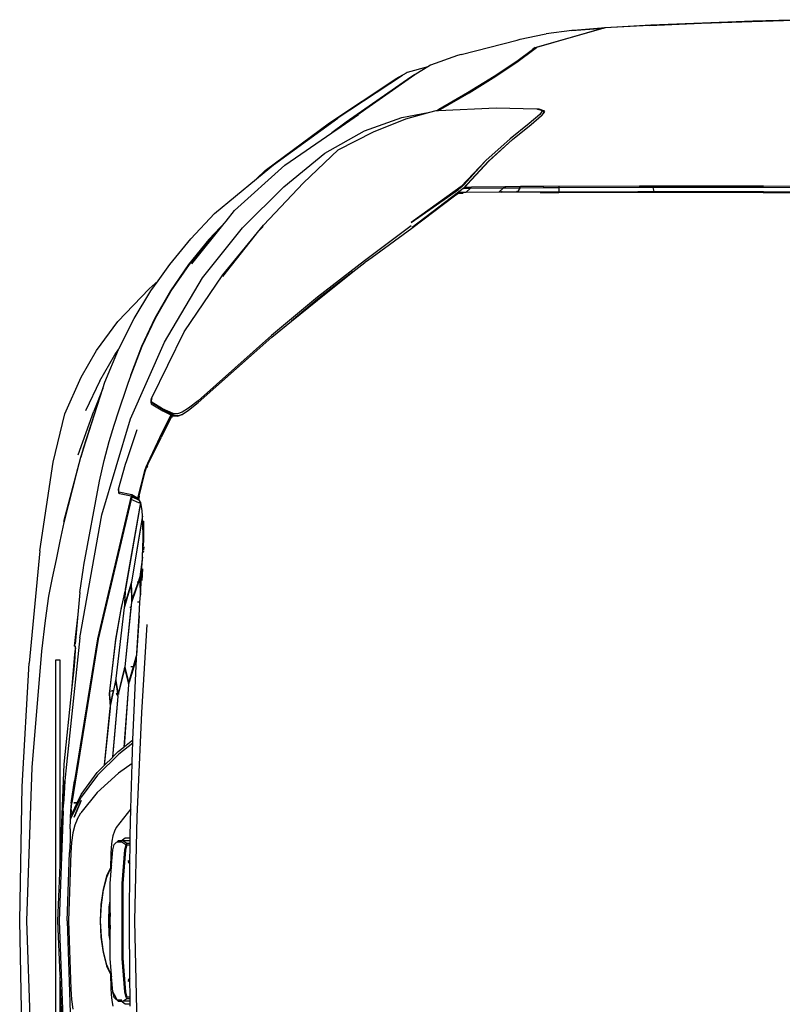
# Model space of a CAD drawing. Units: inches. Extents: x 22042254 to 25404563, y 17568978 to 17626777.
# Tile 12 of 45: x 22042340.5158 to 22042340.9867, y 17568978.1657 to 17568978.7735. Entities that reach past the tile are written whole.
import ezdxf

# ---------------------------------------------------------------- set-up
doc = ezdxf.new("R2010")
doc.units = ezdxf.units.IN
doc.header["$MEASUREMENT"] = 0
doc.layers.add('A-SITE-VEHI', color=8, linetype='Continuous', lineweight=18)
doc.layers.add('Edges', color=250, linetype='Continuous')

# ---------------------------------------------------------------- blocks, each defined once
blk = doc.blocks.new('Nissan Qashqai pl')
at = {"layer": 'Edges'}
for p, q in [((7.32157, 11.66208), (7.32157, 12.18208)), ((7.32607, 12.18208), (7.32607, 11.97794)), ((7.29801, 12.07497), (7.29279, 11.92208)), ((7.33017, 12.07853), (7.32607, 11.97794)), ((7.28835, 12.05625), (7.28572, 11.92208)), ((7.32507, 11.92208), (7.32911, 12.03155)), ((7.40018, 11.92208), (7.40245, 12.02601)), ((7.33294, 11.92208), (7.33653, 12.02372)), ((7.33733, 12.00038), (7.33865, 12.00996)), ((7.37751, 12.0015), (7.37864, 12.00699)), ((7.39589, 12.00706), (7.39588, 12.00508)), ((7.33667, 11.99003), (7.33733, 12.00038)), ((7.37683, 11.99537), (7.37751, 12.0015)), ((7.37985, 11.99831), (7.3787, 11.99283)), ((7.38081, 11.99933), (7.37985, 11.99831)), ((7.38074, 11.99908), (7.37985, 11.99831)), ((7.38002, 11.99534), (7.38305, 12.00106)), ((7.38074, 11.99908), (7.38081, 11.99933)), ((7.38104, 11.99933), (7.38074, 11.99908)), ((7.38081, 11.99933), (7.38402, 12.00208)), ((7.38104, 11.99933), (7.38081, 11.99933)), ((7.38305, 12.00106), (7.38104, 11.99933)), ((7.38659, 12.00106), (7.38305, 12.00106)), ((7.38402, 12.00208), (7.38696, 12.00208)), ((7.38683, 12.00198), (7.38659, 12.00106)), ((7.3875, 12.00106), (7.38659, 12.00106)), ((7.38696, 12.00208), (7.38683, 12.00198)), ((7.39094, 12.00508), (7.38696, 12.00208)), ((7.38696, 12.00208), (7.38847, 12.00208)), ((7.38847, 12.00208), (7.39254, 11.99933)), ((7.39551, 12.00208), (7.38847, 12.00208)), ((7.39041, 11.99283), (7.39156, 11.99831)), ((7.39564, 12.00508), (7.39094, 12.00508)), ((7.39288, 11.99808), (7.39173, 11.99259)), ((7.39254, 11.99933), (7.39582, 11.99933)), ((7.39254, 11.99933), (7.39288, 11.99808)), ((7.3958, 11.99808), (7.39288, 11.99808)), ((7.39551, 12.00208), (7.39584, 12.00183)), ((7.39588, 12.0049), (7.39564, 12.00508)), ((7.39588, 12.00508), (7.39564, 12.00508)), ((7.3958, 11.99808), (7.39564, 11.98012)), ((7.39582, 11.99933), (7.3958, 11.99808)), ((7.39584, 12.00183), (7.39582, 11.99933)), ((7.39588, 12.0049), (7.39584, 12.00183)), ((7.39588, 12.00508), (7.39588, 12.0049)), ((7.33429, 11.92208), (7.33667, 11.99003)), ((7.37614, 11.97511), (7.37648, 11.98901)), ((7.37648, 11.98901), (7.37683, 11.99537)), ((7.3787, 11.99283), (7.37743, 11.97775)), ((7.3787, 11.99283), (7.38002, 11.99534)), ((7.38759, 11.95948), (7.39041, 11.99283)), ((7.39173, 11.99259), (7.38892, 11.95935)), ((7.32607, 11.9764), (7.32607, 11.97794)), ((7.37614, 11.97511), (7.37686, 11.97673)), ((7.37686, 11.97673), (7.3771, 11.97702)), ((7.37713, 11.97709), (7.3771, 11.97702)), ((7.37743, 11.97775), (7.37713, 11.97709)), ((7.37713, 11.97709), (7.3774, 11.97738)), ((7.3774, 11.97738), (7.37727, 11.97594)), ((7.3774, 11.97738), (7.37743, 11.97775)), ((7.39385, 11.98229), (7.39564, 11.98012)), ((7.39563, 11.97885), (7.39385, 11.981)), ((7.39563, 11.97885), (7.3951, 11.92208)), ((7.39564, 11.98012), (7.39563, 11.97885)), ((7.32607, 11.9764), (7.3238, 11.92208)), ((7.37239, 11.9667), (7.37614, 11.97511)), ((7.37707, 11.97569), (7.37268, 11.96585)), ((7.37727, 11.97594), (7.37588, 11.95948)), ((7.37727, 11.97594), (7.37707, 11.97569)), ((7.36896, 11.95363), (7.37239, 11.9667)), ((7.37268, 11.96585), (7.36932, 11.95303)), ((7.37588, 11.95948), (7.37588, 11.94171)), ((7.38759, 11.88468), (7.38759, 11.95948)), ((7.38892, 11.95935), (7.38892, 11.88481)), ((7.36681, 11.93841), (7.36896, 11.95363)), ((7.36932, 11.95303), (7.3672, 11.9381)), ((7.36607, 11.92208), (7.36681, 11.93841)), ((7.3672, 11.9381), (7.36648, 11.92208)), ((7.37588, 11.94171), (7.37512, 11.93632)), ((7.37588, 11.94171), (7.37588, 11.93029)), ((7.37512, 11.93632), (7.37448, 11.92208)), ((7.37551, 11.92208), (7.37588, 11.93029)), ((7.37588, 11.93029), (7.37588, 11.91388)), ((7.28572, 11.92208), (7.28835, 11.78791)), ((7.29279, 11.92208), (7.29801, 11.76919)), ((7.3238, 11.92208), (7.32607, 11.86622)), ((7.32911, 11.81261), (7.32507, 11.92208)), ((7.33294, 11.92208), (7.33535, 11.85392)), ((7.33667, 11.85414), (7.33429, 11.92208)), ((7.36681, 11.90575), (7.36607, 11.92208)), ((7.36648, 11.92208), (7.3672, 11.90606)), ((7.37448, 11.92208), (7.37512, 11.90785)), ((7.37588, 11.91388), (7.37551, 11.92208)), ((7.3951, 11.92208), (7.39563, 11.86531)), ((7.40245, 11.81815), (7.40018, 11.92208)), ((7.37588, 11.91388), (7.37588, 11.90246)), ((7.36896, 11.89053), (7.36681, 11.90575)), ((7.3672, 11.90606), (7.36932, 11.89113)), ((7.37512, 11.90785), (7.37588, 11.90246)), ((7.37588, 11.90246), (7.37588, 11.88468)), ((7.37239, 11.87746), (7.36896, 11.89053)), ((7.36932, 11.89113), (7.37268, 11.87831)), ((7.37588, 11.88468), (7.37727, 11.86822)), ((7.39041, 11.85133), (7.38759, 11.88468)), ((7.38892, 11.88481), (7.39173, 11.85157)), ((7.37614, 11.86905), (7.37239, 11.87746)), ((7.37268, 11.87831), (7.37707, 11.86848)), ((7.37648, 11.85515), (7.37614, 11.86905)), ((7.37686, 11.86743), (7.37614, 11.86905)), ((7.32607, 11.86622), (7.33017, 11.76563)), ((7.32607, 11.86622), (7.32607, 11.66208)), ((7.3771, 11.86714), (7.37686, 11.86743)), ((7.37707, 11.86848), (7.37727, 11.86822)), ((7.3771, 11.86714), (7.37713, 11.86707)), ((7.37713, 11.86707), (7.37743, 11.86641)), ((7.3774, 11.86678), (7.37713, 11.86707)), ((7.37727, 11.86822), (7.3774, 11.86678)), ((7.3774, 11.86678), (7.37743, 11.86641)), ((7.37743, 11.86641), (7.3787, 11.85133)), ((7.39385, 11.86316), (7.39563, 11.86531)), ((7.39564, 11.86404), (7.39385, 11.86187)), ((7.39563, 11.86531), (7.39564, 11.86404)), ((7.39564, 11.86404), (7.3958, 11.84608)), ((7.33608, 11.84164), (7.33535, 11.85392)), ((7.33733, 11.84378), (7.33667, 11.85414)), ((7.37683, 11.8488), (7.37648, 11.85515)), ((7.3787, 11.85133), (7.37985, 11.84585)), ((7.39156, 11.84585), (7.39041, 11.85133)), ((7.39173, 11.85157), (7.39288, 11.84608)), ((7.33619, 11.83012), (7.33608, 11.84164)), ((7.33865, 11.8342), (7.33733, 11.84378)), ((7.37751, 11.84267), (7.37683, 11.8488)), ((7.37864, 11.83717), (7.37751, 11.84267)), ((7.37985, 11.84585), (7.38081, 11.84483)), ((7.38081, 11.84483), (7.38074, 11.84508)), ((7.38081, 11.84483), (7.38104, 11.84483)), ((7.38402, 11.84208), (7.38081, 11.84483)), ((7.38305, 11.8431), (7.3875, 11.8431)), ((7.38696, 11.84208), (7.38402, 11.84208)), ((7.38696, 11.84208), (7.39094, 11.83908)), ((7.38847, 11.84208), (7.38696, 11.84208)), ((7.3875, 11.8431), (7.39156, 11.84585)), ((7.39254, 11.84483), (7.38847, 11.84208)), ((7.39551, 11.84208), (7.38847, 11.84208)), ((7.39288, 11.84608), (7.39254, 11.84483)), ((7.39582, 11.84483), (7.39254, 11.84483)), ((7.39288, 11.84608), (7.3958, 11.84608)), ((7.39584, 11.84233), (7.39551, 11.84208)), ((7.39564, 11.83908), (7.39587, 11.83925)), ((7.3958, 11.84608), (7.39582, 11.84483)), ((7.39582, 11.84483), (7.39584, 11.84233)), ((7.39584, 11.84233), (7.39587, 11.83925)), ((7.39587, 11.83925), (7.39587, 11.83908)), ((7.33619, 11.83012), (7.33653, 11.82044)), ((7.3407, 11.82658), (7.33865, 11.8342)), ((7.38014, 11.8327), (7.37864, 11.83717)), ((7.38184, 11.82907), (7.38014, 11.8327)), ((7.39094, 11.83908), (7.39564, 11.83908)), ((7.39564, 11.83908), (7.39587, 11.83908)), ((7.39587, 11.83908), (7.39589, 11.8371)), ((7.39589, 11.8371), (7.3966, 11.81032)), ((7.33615, 11.81939), (7.33653, 11.82044)), ((7.33672, 11.81955), (7.33615, 11.81939)), ((7.33653, 11.82044), (7.34711, 11.79873)), ((7.34316, 11.82104), (7.3407, 11.82658)), ((7.34316, 11.82104), (7.34679, 11.81424)), ((7.3966, 11.81032), (7.38184, 11.82907)), ((7.32911, 11.81261), (7.32941, 11.80569)), ((7.33645, 11.81201), (7.33615, 11.81939)), ((7.33691, 11.80472), (7.33645, 11.81201)), ((7.33686, 11.81546), (7.33737, 11.81653)), ((7.33691, 11.81132), (7.33686, 11.81546)), ((7.33686, 11.81546), (7.33805, 11.81508)), ((7.33691, 11.81132), (7.33767, 11.80437)), ((7.33737, 11.81653), (7.33805, 11.81508)), ((7.33805, 11.81508), (7.34299, 11.80448)), ((7.34013, 11.81856), (7.34308, 11.8112)), ((7.347, 11.80211), (7.34013, 11.81856)), ((7.34308, 11.8112), (7.347, 11.80211)), ((7.36303, 11.79404), (7.34679, 11.81424)), ((7.3966, 11.81032), (7.39782, 11.76508)), ((7.40723, 11.71423), (7.40245, 11.81815)), ((7.33008, 11.79493), (7.32941, 11.80569)), ((7.3295, 11.80119), (7.33087, 11.78224)), ((7.3295, 11.80119), (7.33008, 11.79493)), ((7.33691, 11.80472), (7.34048, 11.78254)), ((7.33771, 11.80416), (7.33767, 11.80437)), ((7.34104, 11.78371), (7.33771, 11.80416)), ((7.34299, 11.80448), (7.33961, 11.8043)), ((7.33961, 11.8043), (7.34314, 11.80416)), ((7.34299, 11.80448), (7.34314, 11.80416)), ((7.34314, 11.80416), (7.34693, 11.79606)), ((7.33087, 11.78224), (7.33008, 11.79493)), ((7.34693, 11.79606), (7.36309, 11.77403)), ((7.36331, 11.77672), (7.34711, 11.79873)), ((7.38423, 11.77487), (7.36303, 11.79404)), ((7.28835, 11.78791), (7.29513, 11.66508)), ((7.33168, 11.77242), (7.33087, 11.78224)), ((7.36347, 11.6409), (7.34048, 11.78254)), ((7.34263, 11.77348), (7.34104, 11.78371)), ((7.34554, 11.63996), (7.33168, 11.77242)), ((7.36397, 11.64129), (7.34263, 11.77348)), ((7.36309, 11.77403), (7.37008, 11.76708)), ((7.38449, 11.75584), (7.36331, 11.77672)), ((7.39782, 11.76508), (7.38423, 11.77487)), ((7.29801, 11.76919), (7.30777, 11.65317)), ((7.33017, 11.76563), (7.33778, 11.69209)), ((7.37589, 11.71006), (7.37008, 11.76708)), ((7.37008, 11.76708), (7.37036, 11.76681)), ((7.37036, 11.76681), (7.37608, 11.71004)), ((7.37036, 11.76681), (7.37826, 11.75896)), ((7.39782, 11.76508), (7.39816, 11.75211)), ((7.38357, 11.6983), (7.37826, 11.75896)), ((7.37826, 11.75896), (7.37876, 11.75846)), ((7.37876, 11.75846), (7.38403, 11.69824)), ((7.37876, 11.75846), (7.38409, 11.75317)), ((7.38409, 11.75317), (7.38964, 11.74878)), ((7.39848, 11.74482), (7.38449, 11.75584)), ((7.39816, 11.75211), (7.39848, 11.74482)), ((7.39414, 11.68653), (7.38964, 11.74878)), ((7.38964, 11.74878), (7.39027, 11.74828)), ((7.39027, 11.74828), (7.39449, 11.68648)), ((7.39027, 11.74828), (7.39862, 11.74167)), ((7.39848, 11.74482), (7.39862, 11.74167)), ((7.39862, 11.74167), (7.40182, 11.66777)), ((7.41241, 11.62655), (7.40723, 11.71423)), ((7.37498, 11.69572), (7.37596, 11.70814)), ((7.37623, 11.70617), (7.37575, 11.69593)), ((7.37596, 11.70814), (7.37589, 11.71006)), ((7.37608, 11.71004), (7.37634, 11.7081)), ((7.37623, 11.70617), (7.37642, 11.70614)), ((7.37634, 11.7081), (7.38127, 11.68424)), ((7.37642, 11.70614), (7.37916, 11.6924)), ((7.33778, 11.69209), (7.34072, 11.65629)), ((7.33778, 11.69209), (7.33996, 11.67104)), ((7.38128, 11.64204), (7.37498, 11.69572)), ((7.37575, 11.69593), (7.37562, 11.69326)), ((7.37916, 11.6924), (7.37562, 11.69326)), ((7.37562, 11.69326), (7.38154, 11.64126)), ((7.37568, 11.69592), (7.37575, 11.69593)), ((7.38118, 11.68226), (7.37916, 11.6924)), ((7.38174, 11.68442), (7.38322, 11.69486)), ((7.38379, 11.69443), (7.38202, 11.68226)), ((7.38243, 11.69547), (7.38357, 11.6983)), ((7.3835, 11.69733), (7.38243, 11.69547)), ((7.38336, 11.69586), (7.38243, 11.69547)), ((7.38243, 11.69547), (7.38322, 11.69486)), ((7.38324, 11.69498), (7.38243, 11.69547)), ((7.38322, 11.69486), (7.38379, 11.69443)), ((7.38324, 11.69498), (7.38336, 11.69586)), ((7.38377, 11.69466), (7.38324, 11.69498)), ((7.3837, 11.696), (7.38336, 11.69586)), ((7.3835, 11.69733), (7.38357, 11.6983)), ((7.38361, 11.69752), (7.3835, 11.69733)), ((7.38361, 11.69752), (7.38357, 11.6983)), ((7.38403, 11.69824), (7.38361, 11.69752)), ((7.38438, 11.69629), (7.3837, 11.696)), ((7.38377, 11.69466), (7.3837, 11.696)), ((7.38426, 11.69437), (7.38377, 11.69466)), ((7.38429, 11.69425), (7.38379, 11.69443)), ((7.38426, 11.69437), (7.38438, 11.69629)), ((7.38429, 11.69425), (7.38426, 11.69437)), ((7.38773, 11.68027), (7.38429, 11.69425)), ((7.38438, 11.69629), (7.39028, 11.67251)), ((7.38152, 11.68035), (7.38118, 11.68226)), ((7.38127, 11.68424), (7.38174, 11.68442)), ((7.3817, 11.68412), (7.38127, 11.68424)), ((7.3817, 11.68412), (7.38174, 11.68442)), ((7.38202, 11.68226), (7.38195, 11.68031)), ((7.39093, 11.67275), (7.39387, 11.6846)), ((7.39425, 11.68274), (7.39127, 11.6705)), ((7.39387, 11.6846), (7.39414, 11.68653)), ((7.39425, 11.68274), (7.39494, 11.68257)), ((7.39425, 11.68274), (7.39497, 11.68247)), ((7.39449, 11.68648), (7.39509, 11.68353)), ((7.39497, 11.68247), (7.39494, 11.68257)), ((7.39898, 11.66858), (7.39497, 11.68247)), ((7.39509, 11.68353), (7.40207, 11.66087)), ((7.38995, 11.60941), (7.38152, 11.68035)), ((7.38195, 11.68031), (7.39032, 11.60945)), ((7.38737, 11.68027), (7.38773, 11.68027)), ((7.39008, 11.67074), (7.38773, 11.68027)), ((7.39093, 11.67275), (7.39028, 11.67251)), ((7.39087, 11.67252), (7.39028, 11.67251)), ((7.39087, 11.67252), (7.39093, 11.67275)), ((7.3059, 11.55319), (7.29513, 11.66508)), ((7.33996, 11.67104), (7.34097, 11.65941)), ((7.39046, 11.66873), (7.39008, 11.67074)), ((7.3966, 11.6095), (7.39046, 11.66873)), ((7.39127, 11.6705), (7.39107, 11.66865)), ((7.39107, 11.66865), (7.39768, 11.60417)), ((7.39898, 11.66858), (7.39666, 11.66858)), ((7.4017, 11.65916), (7.39898, 11.66858)), ((7.40182, 11.66777), (7.40224, 11.66093)), ((7.30777, 11.65317), (7.31133, 11.62243)), ((7.32607, 11.66208), (7.32157, 11.66208)), ((7.34072, 11.65629), (7.34131, 11.65087)), ((7.34097, 11.65941), (7.34133, 11.65108)), ((7.40216, 11.65713), (7.4017, 11.65916)), ((7.40224, 11.66093), (7.40207, 11.66087)), ((7.40224, 11.66086), (7.40207, 11.66087)), ((7.40484, 11.618), (7.40216, 11.65713)), ((7.40224, 11.66093), (7.40224, 11.66086)), ((7.40224, 11.66086), (7.40484, 11.618)), ((7.34009, 11.64801), (7.34004, 11.64799)), ((7.3438, 11.61665), (7.34004, 11.64799)), ((7.34097, 11.64796), (7.34009, 11.64801)), ((7.34097, 11.64796), (7.34131, 11.65087)), ((7.34097, 11.64796), (7.34145, 11.64799)), ((7.34144, 11.64796), (7.34097, 11.64796)), ((7.3438, 11.61665), (7.34121, 11.64598)), ((7.34133, 11.65108), (7.34131, 11.65087)), ((7.34131, 11.65087), (7.34154, 11.6488)), ((7.34554, 11.63996), (7.36761, 11.51724)), ((7.39705, 11.49808), (7.36347, 11.6409)), ((7.39678, 11.50175), (7.36397, 11.64129)), ((7.3869, 11.60943), (7.38128, 11.64204)), ((7.38154, 11.64126), (7.38644, 11.61311)), ((7.31133, 11.62243), (7.31494, 11.59842)), ((7.34574, 11.59466), (7.3438, 11.61665)), ((7.40484, 11.618), (7.40567, 11.60418)), ((7.38644, 11.61311), (7.39089, 11.59332)), ((7.39116, 11.59143), (7.3869, 11.60943)), ((7.39012, 11.60735), (7.38995, 11.60941)), ((7.39099, 11.59348), (7.39012, 11.60735)), ((7.39032, 11.60945), (7.3908, 11.60755)), ((7.39058, 11.60552), (7.39095, 11.60545)), ((7.39058, 11.60552), (7.39098, 11.60538)), ((7.39058, 11.60552), (7.39141, 11.59144)), ((7.3908, 11.60755), (7.39654, 11.58812)), ((7.39098, 11.60538), (7.39095, 11.60545)), ((7.39668, 11.58624), (7.39098, 11.60538)), ((7.3966, 11.6095), (7.39566, 11.6095)), ((7.39715, 11.60416), (7.3966, 11.6095)), ((7.39722, 11.60211), (7.39715, 11.60416)), ((7.39768, 11.60417), (7.39823, 11.60225)), ((7.40567, 11.60418), (7.40319, 11.60418)), ((7.40567, 11.60418), (7.40611, 11.59696)), ((7.31494, 11.59842), (7.3186, 11.58002)), ((7.34574, 11.59466), (7.34938, 11.57004)), ((7.39684, 11.58823), (7.39722, 11.60211)), ((7.39774, 11.60029), (7.39733, 11.58621)), ((7.39774, 11.60029), (7.39827, 11.60018)), ((7.39774, 11.60029), (7.39831, 11.60008)), ((7.39823, 11.60225), (7.40485, 11.58292)), ((7.39831, 11.60008), (7.39827, 11.60018)), ((7.40376, 11.5843), (7.39831, 11.60008)), ((7.40533, 11.58312), (7.40611, 11.59688)), ((7.40611, 11.59688), (7.40611, 11.59696)), ((7.40611, 11.59688), (7.40642, 11.59185)), ((7.39099, 11.59348), (7.39089, 11.59332)), ((7.39101, 11.59337), (7.39089, 11.59332)), ((7.39156, 11.58943), (7.39116, 11.59143)), ((7.39141, 11.59144), (7.39169, 11.5895)), ((7.40622, 11.5053), (7.39156, 11.58943)), ((7.39169, 11.5895), (7.40648, 11.50498)), ((7.39684, 11.58823), (7.39654, 11.58812)), ((7.39714, 11.58424), (7.39668, 11.58624)), ((7.39684, 11.58823), (7.39731, 11.58844)), ((7.40828, 11.51835), (7.39714, 11.58424)), ((7.39733, 11.58621), (7.39747, 11.58427)), ((7.39747, 11.58427), (7.40836, 11.51976)), ((7.40376, 11.5843), (7.40279, 11.5843)), ((7.40488, 11.58107), (7.40376, 11.5843)), ((7.40642, 11.59185), (7.40597, 11.58338)), ((7.40642, 11.59185), (7.40687, 11.58436)), ((7.40687, 11.58436), (7.40791, 11.56437)), ((7.3186, 11.58002), (7.32232, 11.56164)), ((7.40533, 11.58312), (7.40485, 11.58292)), ((7.40532, 11.58299), (7.40485, 11.58292)), ((7.40539, 11.57906), (7.40488, 11.58107)), ((7.40597, 11.58327), (7.40532, 11.58299)), ((7.40532, 11.58299), (7.40533, 11.58312)), ((7.40597, 11.58338), (7.40533, 11.58312)), ((7.40814, 11.55935), (7.40539, 11.57906)), ((7.40597, 11.58327), (7.40585, 11.58097)), ((7.40585, 11.58097), (7.40588, 11.57905)), ((7.40588, 11.57905), (7.40791, 11.56437)), ((7.40597, 11.58338), (7.40597, 11.58327)), ((7.40813, 11.57111), (7.40752, 11.58276)), ((7.34938, 11.57004), (7.3497, 11.56742)), ((7.34938, 11.57004), (7.34978, 11.56736)), ((7.3497, 11.56742), (7.36534, 11.48377)), ((7.40791, 11.56437), (7.40811, 11.56038)), ((7.40791, 11.56437), (7.40812, 11.56285)), ((7.32232, 11.56164), (7.3261, 11.54328)), ((7.40811, 11.56038), (7.40814, 11.55935)), ((7.40814, 11.55935), (7.40871, 11.54047)), ((7.40926, 11.55458), (7.40949, 11.55292)), ((7.3059, 11.55319), (7.31925, 11.46451)), ((7.40923, 11.54161), (7.40902, 11.54853)), ((7.4096, 11.54898), (7.40916, 11.55209)), ((7.3261, 11.54328), (7.32996, 11.52493)), ((7.40871, 11.54047), (7.40865, 11.52464)), ((7.40921, 11.52579), (7.40923, 11.54161)), ((7.40908, 11.52353), (7.40921, 11.52579)), ((7.3297, 11.52373), (7.34671, 11.45961)), ((7.32996, 11.52493), (7.34671, 11.45961)), ((7.36761, 11.51724), (7.39627, 11.42146)), ((7.40828, 11.51835), (7.40795, 11.51289)), ((7.40836, 11.51976), (7.40828, 11.51835)), ((7.40865, 11.52464), (7.40836, 11.51976)), ((7.40795, 11.51289), (7.4066, 11.50521)), ((7.38529, 11.49584), (7.38412, 11.49562)), ((7.38437, 11.49158), (7.38412, 11.49562)), ((7.39764, 11.49714), (7.38458, 11.49463)), ((7.38529, 11.49584), (7.38458, 11.49463)), ((7.38529, 11.49584), (7.39705, 11.49808)), ((7.40464, 11.5053), (7.39678, 11.50175)), ((7.39804, 11.49925), (7.39678, 11.50175)), ((7.39705, 11.49808), (7.39833, 11.49833)), ((7.40264, 11.50022), (7.39764, 11.49714)), ((7.39804, 11.49925), (7.40478, 11.50242)), ((7.4012, 11.50009), (7.39804, 11.49925)), ((7.39833, 11.49833), (7.4012, 11.50009)), ((7.4012, 11.50009), (7.40335, 11.50141)), ((7.40299, 11.50047), (7.40264, 11.50022)), ((7.40299, 11.50047), (7.40276, 11.50042)), ((7.40326, 11.50066), (7.40299, 11.50047)), ((7.40417, 11.50199), (7.40326, 11.50066)), ((7.4033, 11.50053), (7.40326, 11.50066)), ((7.40335, 11.50054), (7.4033, 11.50053)), ((7.41007, 11.47333), (7.4033, 11.50053)), ((7.40335, 11.50141), (7.40417, 11.50199)), ((7.40425, 11.50164), (7.40405, 11.50122)), ((7.40431, 11.5014), (7.40405, 11.50122)), ((7.40405, 11.50122), (7.41077, 11.47382)), ((7.40417, 11.50199), (7.40443, 11.50199)), ((7.40425, 11.50164), (7.40417, 11.50199)), ((7.40443, 11.50199), (7.40425, 11.50164)), ((7.40431, 11.5014), (7.40425, 11.50164)), ((7.40461, 11.50161), (7.40431, 11.5014)), ((7.40447, 11.50076), (7.40431, 11.5014)), ((7.40456, 11.50227), (7.40443, 11.50199)), ((7.40443, 11.50199), (7.40463, 11.50199)), ((7.4048, 11.50082), (7.40447, 11.50076)), ((7.40502, 11.49854), (7.40447, 11.50076)), ((7.40456, 11.50227), (7.40478, 11.50242)), ((7.40497, 11.50227), (7.40456, 11.50227)), ((7.40456, 11.50227), (7.40463, 11.50199)), ((7.40469, 11.50176), (7.40461, 11.50161)), ((7.40463, 11.50199), (7.40469, 11.50176)), ((7.40463, 11.50199), (7.40482, 11.50199)), ((7.40622, 11.5053), (7.40464, 11.5053)), ((7.40482, 11.50199), (7.40469, 11.50176)), ((7.40478, 11.50242), (7.40523, 11.50274)), ((7.40515, 11.5026), (7.40478, 11.50242)), ((7.40497, 11.50227), (7.40482, 11.50199)), ((7.40515, 11.5026), (7.40497, 11.50227)), ((7.40523, 11.50274), (7.40515, 11.5026)), ((7.40632, 11.5047), (7.40523, 11.50274)), ((7.40632, 11.5047), (7.40622, 11.5053)), ((7.40648, 11.50498), (7.40632, 11.5047)), ((7.4066, 11.50521), (7.40648, 11.50498)), ((7.38458, 11.49463), (7.38437, 11.49158)), ((7.38437, 11.49158), (7.39136, 11.46669)), ((7.36534, 11.48377), (7.36995, 11.46286)), ((7.39136, 11.46669), (7.39248, 11.46286)), ((7.41147, 11.46951), (7.41007, 11.47333)), ((7.41077, 11.47382), (7.41219, 11.47)), ((7.41315, 11.46587), (7.41147, 11.46951)), ((7.41219, 11.47), (7.41393, 11.46637)), ((7.41256, 11.46999), (7.41248, 11.47021)), ((7.41324, 11.46853), (7.41256, 11.46999)), ((7.41393, 11.46637), (7.42672, 11.44006)), ((7.31925, 11.46451), (7.3309, 11.41659)), ((7.34401, 11.45722), (7.35959, 11.41392)), ((7.34891, 11.45171), (7.34671, 11.45961)), ((7.34671, 11.45961), (7.36864, 11.39135)), ((7.36995, 11.46286), (7.375, 11.44419)), ((7.39248, 11.46286), (7.39374, 11.45905)), ((7.39374, 11.45905), (7.40289, 11.43211)), ((7.42553, 11.43981), (7.41315, 11.46587)), ((7.34891, 11.45171), (7.36864, 11.39135)), ((7.375, 11.44419), (7.37986, 11.42777)), ((7.42553, 11.43981), (7.43673, 11.41738)), ((7.43787, 11.41791), (7.42672, 11.44006)), ((7.37986, 11.42777), (7.38454, 11.41358)), ((7.39627, 11.42146), (7.43015, 11.3449)), ((7.43587, 11.41698), (7.43673, 11.41738)), ((7.43832, 11.417), (7.43673, 11.41738)), ((7.43751, 11.42004), (7.43844, 11.41817)), ((7.43787, 11.41791), (7.43844, 11.41817)), ((7.4389, 11.41727), (7.43787, 11.41791)), ((7.43832, 11.417), (7.43787, 11.41791)), ((7.4389, 11.41727), (7.43832, 11.417)), ((7.43844, 11.41817), (7.43873, 11.41831)), ((7.43873, 11.41831), (7.44298, 11.41881)), ((7.4389, 11.41727), (7.44004, 11.41781)), ((7.44418, 11.41831), (7.44004, 11.41781)), ((7.44298, 11.41881), (7.44771, 11.41717)), ((7.44771, 11.41717), (7.44418, 11.41831)), ((7.44771, 11.41717), (7.45415, 11.41285)), ((7.3309, 11.41659), (7.34698, 11.37976)), ((7.36552, 11.38372), (7.3514, 11.41334)), ((7.36864, 11.39135), (7.35959, 11.41392)), ((7.38454, 11.41358), (7.39247, 11.38995)), ((7.42821, 11.41133), (7.41689, 11.40438)), ((7.41697, 11.40649), (7.42833, 11.41346)), ((7.42961, 11.41292), (7.4183, 11.40596)), ((7.43873, 11.41619), (7.42821, 11.41133)), ((7.42833, 11.41346), (7.43587, 11.41698)), ((7.42961, 11.41292), (7.43832, 11.417)), ((7.44309, 11.41655), (7.43873, 11.41619)), ((7.44789, 11.41487), (7.44309, 11.41655)), ((7.4541, 11.41081), (7.44789, 11.41487)), ((7.46355, 11.40337), (7.4541, 11.41081)), ((7.45415, 11.41285), (7.46382, 11.40513)), ((7.41665, 11.40488), (7.41697, 11.40649)), ((7.41716, 11.40469), (7.41665, 11.40488)), ((7.41687, 11.40359), (7.41665, 11.40488)), ((7.41687, 11.40359), (7.41686, 11.40296)), ((7.41686, 11.40296), (7.41723, 11.40107)), ((7.41689, 11.40438), (7.41687, 11.40359)), ((7.41717, 11.40184), (7.41687, 11.40359)), ((7.41716, 11.40469), (7.41689, 11.40438)), ((7.4183, 11.40596), (7.41716, 11.40469)), ((7.41744, 11.4013), (7.41717, 11.40184)), ((7.41723, 11.40107), (7.44978, 11.33488)), ((7.41744, 11.4013), (7.41747, 11.40124)), ((7.53689, 11.33848), (7.46355, 11.40337)), ((7.46382, 11.40513), (7.53708, 11.33997)), ((7.36864, 11.39135), (7.37074, 11.38491)), ((7.39247, 11.38995), (7.39379, 11.3859)), ((7.34698, 11.37976), (7.36237, 11.35349)), ((7.36552, 11.38372), (7.38053, 11.35758)), ((7.37074, 11.38491), (7.38426, 11.35219)), ((7.39379, 11.3859), (7.39513, 11.38217)), ((7.39513, 11.38217), (7.39648, 11.37869)), ((7.39621, 11.37814), (7.39648, 11.37869)), ((7.40715, 11.34933), (7.39621, 11.37814)), ((7.39648, 11.37869), (7.39687, 11.3777)), ((7.39687, 11.3777), (7.40781, 11.34902)), ((7.36237, 11.35349), (7.38367, 11.32447)), ((7.38053, 11.35758), (7.38426, 11.35219)), ((7.38426, 11.35219), (7.38446, 11.35171)), ((7.38446, 11.35171), (7.39973, 11.32146)), ((7.42053, 11.32124), (7.40715, 11.34933)), ((7.40781, 11.34902), (7.42115, 11.32101)), ((7.43015, 11.3449), (7.46788, 11.28072)), ((7.58274, 11.30006), (7.53689, 11.33848)), ((7.53708, 11.33997), (7.55684, 11.32404)), ((7.44978, 11.33488), (7.48836, 11.27781)), ((7.38367, 11.32447), (7.41469, 11.29179)), ((7.39973, 11.32146), (7.41661, 11.29389)), ((7.43626, 11.29398), (7.42053, 11.32124)), ((7.42115, 11.32101), (7.4369, 11.29377)), ((7.58398, 11.30127), (7.55684, 11.32404)), ((7.55684, 11.32404), (7.58288, 11.30303)), ((7.6296, 11.2639), (7.58274, 11.30006)), ((7.58288, 11.30303), (7.61803, 11.27504)), ((7.61803, 11.27504), (7.58398, 11.30127)), ((7.41469, 11.29179), (7.42386, 11.28371)), ((7.41661, 11.29389), (7.42386, 11.28371)), ((7.45423, 11.26769), (7.43626, 11.29398)), ((7.4369, 11.29377), (7.45491, 11.26748)), ((7.42386, 11.28371), (7.4354, 11.26752)), ((7.46788, 11.28072), (7.50805, 11.2311)), ((7.48817, 11.27966), (7.52431, 11.23409)), ((7.48836, 11.27781), (7.52891, 11.22832)), ((7.61803, 11.27504), (7.63007, 11.26544)), ((7.4354, 11.26752), (7.45654, 11.24186)), ((7.47438, 11.24268), (7.45423, 11.26769)), ((7.45491, 11.26748), (7.47504, 11.24255)), ((7.45735, 11.26699), (7.48846, 11.22834)), ((7.67598, 11.22893), (7.6296, 11.2639)), ((7.63007, 11.26544), (7.63056, 11.26506)), ((7.63056, 11.26506), (7.63059, 11.26504)), ((7.63059, 11.26504), (7.6373, 11.26013)), ((7.6373, 11.26013), (7.67691, 11.23122)), ((7.45654, 11.24186), (7.48015, 11.2168)), ((7.49177, 11.22424), (7.47438, 11.24268)), ((7.47504, 11.24255), (7.47703, 11.24044)), ((7.47703, 11.24044), (7.47653, 11.24106)), ((7.47703, 11.24053), (7.47751, 11.23993)), ((7.47838, 11.23878), (7.47703, 11.24044)), ((7.47703, 11.24044), (7.47751, 11.23993)), ((7.47751, 11.23993), (7.47871, 11.23847)), ((7.47751, 11.23993), (7.47869, 11.23868)), ((7.47869, 11.23868), (7.47824, 11.23925)), ((7.4795, 11.2377), (7.47869, 11.23868)), ((7.47869, 11.23868), (7.48846, 11.22834)), ((7.50805, 11.2311), (7.5492, 11.19016)), ((7.52431, 11.23409), (7.52857, 11.22958)), ((7.67691, 11.23122), (7.71943, 11.19922)), ((7.72318, 11.19554), (7.67713, 11.2307)), ((7.48846, 11.22834), (7.49177, 11.22424)), ((7.49177, 11.22424), (7.50008, 11.21391)), ((7.52891, 11.22832), (7.56866, 11.18624)), ((7.72614, 11.18985), (7.67617, 11.22557)), ((7.67617, 11.22557), (7.72327, 11.1928)), ((7.48015, 11.2168), (7.52174, 11.18228)), ((7.50008, 11.21391), (7.55011, 11.16843)), ((7.71943, 11.19922), (7.72318, 11.19658)), ((7.72318, 11.19658), (7.72785, 11.19647)), ((7.72807, 11.19181), (7.72318, 11.19554)), ((7.72318, 11.19554), (7.72455, 11.19553)), ((7.72667, 11.19023), (7.72327, 11.1928)), ((7.72467, 11.19542), (7.72455, 11.19553)), ((7.72455, 11.19553), (7.72942, 11.19548)), ((7.72807, 11.19181), (7.72986, 11.19044)), ((7.73491, 11.19175), (7.72807, 11.19181)), ((7.75301, 11.16475), (7.72807, 11.19181)), ((7.72942, 11.19548), (7.73096, 11.19549)), ((7.73096, 11.19549), (7.73491, 11.19175)), ((7.73096, 11.19549), (7.76399, 11.19528)), ((7.76799, 11.19147), (7.73491, 11.19175)), ((7.76399, 11.19528), (7.7636, 11.19566)), ((7.76799, 11.19147), (7.76399, 11.19528)), ((7.76399, 11.19528), (7.76622, 11.19527)), ((7.76586, 11.19567), (7.76622, 11.19527)), ((7.76622, 11.19527), (7.76683, 11.19458)), ((7.76622, 11.19527), (7.78115, 11.19519)), ((7.76925, 11.19146), (7.76799, 11.19147)), ((7.78439, 11.19133), (7.76925, 11.19146)), ((7.78115, 11.19519), (7.78091, 11.19575)), ((7.7814, 11.19458), (7.78115, 11.19519)), ((7.78115, 11.19519), (7.78224, 11.19518)), ((7.78224, 11.19518), (7.78192, 11.19576)), ((7.78224, 11.19518), (7.80566, 11.19505)), ((7.78439, 11.19133), (7.78224, 11.19518)), ((7.80777, 11.19113), (7.78439, 11.19133)), ((7.80482, 11.19588), (7.82329, 11.1958)), ((7.80566, 11.19505), (7.82329, 11.19498)), ((7.82329, 11.19498), (7.82329, 11.1958)), ((7.82329, 11.1958), (7.90142, 11.19549)), ((7.82329, 11.19498), (7.90204, 11.19468)), ((7.82329, 11.19107), (7.82329, 11.19498)), ((7.90142, 11.19549), (7.91849, 11.19552)), ((7.90204, 11.19468), (7.91833, 11.1947)), ((7.91833, 11.1947), (7.9176, 11.19075)), ((7.91849, 11.19552), (7.91833, 11.1947)), ((7.91833, 11.1947), (8.02749, 11.19482)), ((7.91849, 11.19552), (8.02732, 11.19568)), ((8.02732, 11.19568), (8.17527, 11.1963)), ((8.02749, 11.19482), (8.08756, 11.19507)), ((7.53043, 11.17373), (7.52174, 11.18228)), ((7.52174, 11.18228), (7.53868, 11.16822)), ((7.5492, 11.19016), (7.58999, 11.1565)), ((7.56866, 11.18624), (7.60319, 11.15334)), ((7.72614, 11.18985), (7.75074, 11.16383)), ((7.72856, 11.18809), (7.72667, 11.19023)), ((7.75074, 11.16383), (7.72856, 11.18809)), ((7.72986, 11.19044), (7.73238, 11.18764)), ((7.72986, 11.19044), (7.73635, 11.19039)), ((7.73238, 11.18764), (7.75388, 11.16419)), ((7.7363, 11.19044), (7.73635, 11.19039)), ((7.76942, 11.19011), (7.73635, 11.19039)), ((7.76942, 11.19011), (7.76874, 11.19075)), ((7.7707, 11.1901), (7.76942, 11.19011)), ((7.78514, 11.18998), (7.7707, 11.1901)), ((7.78462, 11.19091), (7.78514, 11.18998)), ((7.80829, 11.18979), (7.78514, 11.18998)), ((7.82329, 11.19107), (7.80777, 11.19113)), ((7.90396, 11.18944), (7.80829, 11.18979)), ((7.82329, 11.18994), (7.82329, 11.19107)), ((7.90357, 11.19074), (7.82329, 11.19107)), ((7.9176, 11.19075), (7.90357, 11.19074)), ((8.02759, 11.18962), (7.90396, 11.18944)), ((8.0275, 11.19086), (7.9176, 11.19075)), ((8.08729, 11.1911), (8.0275, 11.19086)), ((8.17534, 11.1903), (8.02759, 11.18962)), ((7.53043, 11.17373), (7.59458, 11.12619)), ((7.53868, 11.16822), (7.60312, 11.12171)), ((7.55011, 11.16843), (7.59689, 11.13645)), ((7.77477, 11.14231), (7.75074, 11.16383)), ((7.75301, 11.16475), (7.77724, 11.14311)), ((7.75388, 11.16419), (7.77724, 11.14311)), ((7.58999, 11.1565), (7.62951, 11.13442)), ((7.60319, 11.15334), (7.63858, 11.13525)), ((7.79381, 11.1271), (7.77477, 11.14231)), ((7.77724, 11.14311), (7.79586, 11.12808)), ((7.61132, 11.12557), (7.59689, 11.13645)), ((7.59689, 11.13645), (7.6021, 11.13289)), ((7.6021, 11.13289), (7.61183, 11.12554)), ((7.6021, 11.13289), (7.62368, 11.11814)), ((7.62951, 11.13442), (7.66697, 11.12116)), ((7.63858, 11.13525), (7.67084, 11.12249)), ((7.59458, 11.12619), (7.66077, 11.0825)), ((7.67585, 11.08087), (7.61132, 11.12557)), ((7.61183, 11.12554), (7.67993, 11.07831)), ((7.80447, 11.11791), (7.79381, 11.1271)), ((7.79586, 11.12808), (7.80619, 11.11916)), ((7.66763, 11.07907), (7.60245, 11.12206)), ((7.66697, 11.12116), (7.69488, 11.11584)), ((7.67084, 11.12249), (7.69488, 11.11584)), ((7.69488, 11.11584), (7.70101, 11.11415)), ((7.70101, 11.11415), (7.70235, 11.11408)), ((7.70382, 11.11316), (7.70235, 11.11408)), ((7.70235, 11.11408), (7.70343, 11.11403)), ((7.70343, 11.11403), (7.70559, 11.11279)), ((7.70343, 11.11403), (7.76082, 11.11124)), ((7.73247, 11.09659), (7.70382, 11.11316)), ((7.70559, 11.11279), (7.73411, 11.09632)), ((7.80216, 11.1126), (7.80721, 11.11412)), ((7.80956, 11.11476), (7.80372, 11.11265)), ((7.80721, 11.11412), (7.80447, 11.11791)), ((7.80867, 11.11585), (7.80619, 11.11916)), ((7.80619, 11.11916), (7.80665, 11.11877)), ((7.80665, 11.11877), (7.80956, 11.11476)), ((7.80721, 11.11412), (7.80867, 11.11585)), ((7.76082, 11.11124), (7.80143, 11.11238)), ((7.80143, 11.11238), (7.80216, 11.1126)), ((7.80372, 11.11265), (7.80216, 11.1126)), ((7.75906, 11.08002), (7.73247, 11.09659)), ((7.73411, 11.09632), (7.76061, 11.0798)), ((7.67122, 11.0767), (7.66077, 11.0825)), ((7.67207, 11.07622), (7.67122, 11.0767)), ((7.6926, 11.07047), (7.67207, 11.07622)), ((7.67933, 11.07844), (7.67585, 11.08087)), ((7.68018, 11.07816), (7.67933, 11.07844)), ((7.68018, 11.07816), (7.67993, 11.07831)), ((7.68089, 11.07772), (7.68018, 11.07816)), ((7.6926, 11.07047), (7.68089, 11.07772)), ((7.78138, 11.06503), (7.75906, 11.08002)), ((7.76061, 11.0798), (7.78285, 11.06486)), ((7.69527, 11.06881), (7.6926, 11.07047)), ((7.72226, 11.05905), (7.69527, 11.06881)), ((7.79699, 11.05342), (7.78138, 11.06503)), ((7.78285, 11.06486), (7.79842, 11.05331)), ((7.72615, 11.0581), (7.72226, 11.05905)), ((7.72615, 11.0581), (7.78191, 11.04384)), ((7.79699, 11.05342), (7.79703, 11.05339)), ((7.79979, 11.05134), (7.79703, 11.05339)), ((7.79842, 11.05331), (7.80074, 11.05158)), ((7.79979, 11.05134), (7.86763, 11.03183)), ((7.80074, 11.05158), (7.80015, 11.05168)), ((7.80074, 11.05158), (7.80119, 11.05125)), ((7.86805, 11.03202), (7.80119, 11.05125)), ((7.78191, 11.04384), (7.78484, 11.043)), ((7.78484, 11.043), (7.80866, 11.03796)), ((7.80866, 11.03796), (7.81062, 11.03771)), ((7.81073, 11.03768), (7.81062, 11.03771)), ((7.83626, 11.03444), (7.81073, 11.03768)), ((7.83812, 11.0342), (7.83626, 11.03444)), ((7.83626, 11.03444), (7.86763, 11.03183)), ((7.86997, 11.03154), (7.83812, 11.0342)), ((7.86805, 11.03202), (7.86763, 11.03183)), ((7.86805, 11.03202), (7.86903, 11.03174)), ((7.91369, 11.02919), (7.86903, 11.03174)), ((7.91514, 11.02896), (7.86997, 11.03154)), ((7.91369, 11.02919), (7.96577, 11.02701)), ((7.96683, 11.02681), (7.91514, 11.02896)), ((7.96577, 11.02701), (8.01597, 11.02528)), ((8.01677, 11.0251), (7.96683, 11.02681)), ((8.01597, 11.02528), (8.07131, 11.02365)), ((8.07176, 11.02351), (8.01677, 11.0251))]:
    blk.add_line(p, q, dxfattribs=at)
blk = doc.blocks.new('CAR')
blk.add_blockref('Nissan Qashqai pl', (-9.74328, -11.91512))

msp = doc.modelspace()

# ---------------------------------------------------------------- block references
at = {"layer": 'A-SITE-VEHI', "xscale": -0.6191396643141144, "yscale": 0.6191396643141144, "zscale": 0.6191396643141144, "rotation": 180}
msp.add_blockref('CAR', (22042342.03736, 17568978.22147), dxfattribs=at)

doc.saveas('drawing.dxf')
